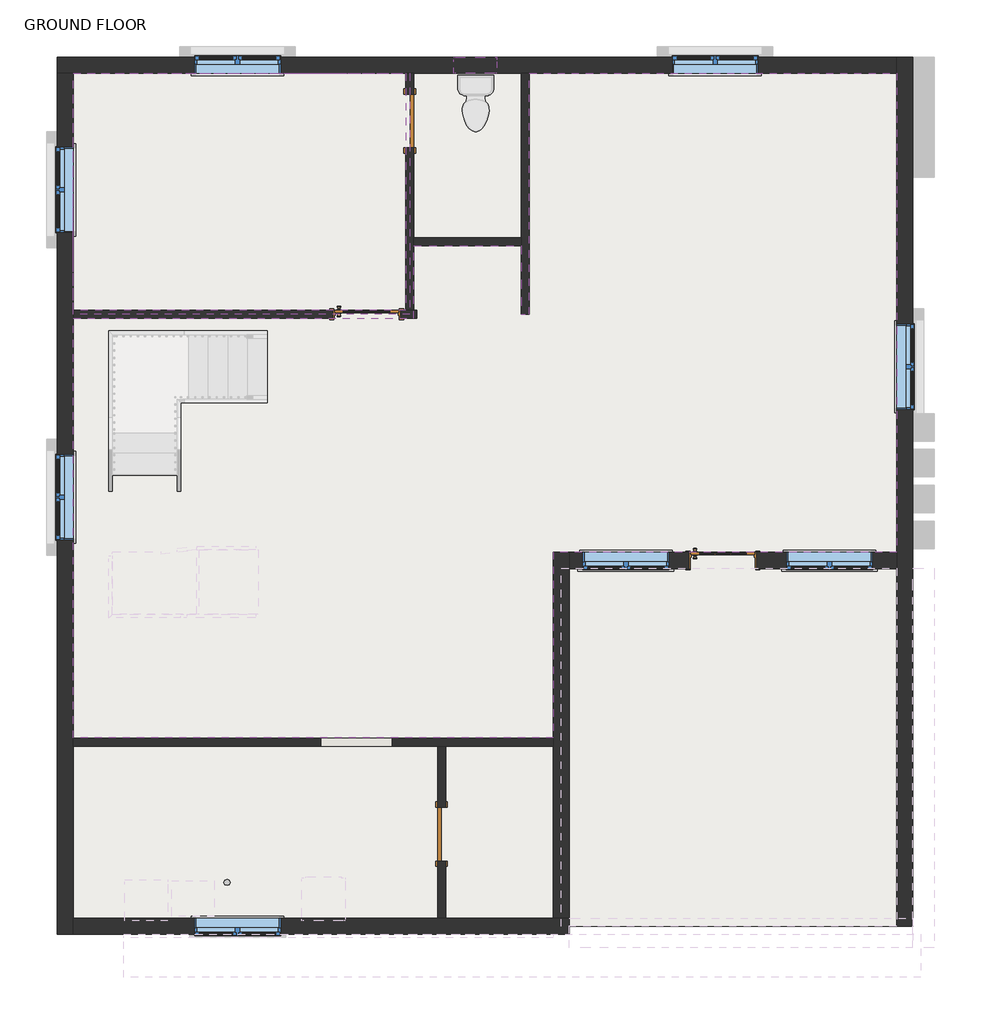
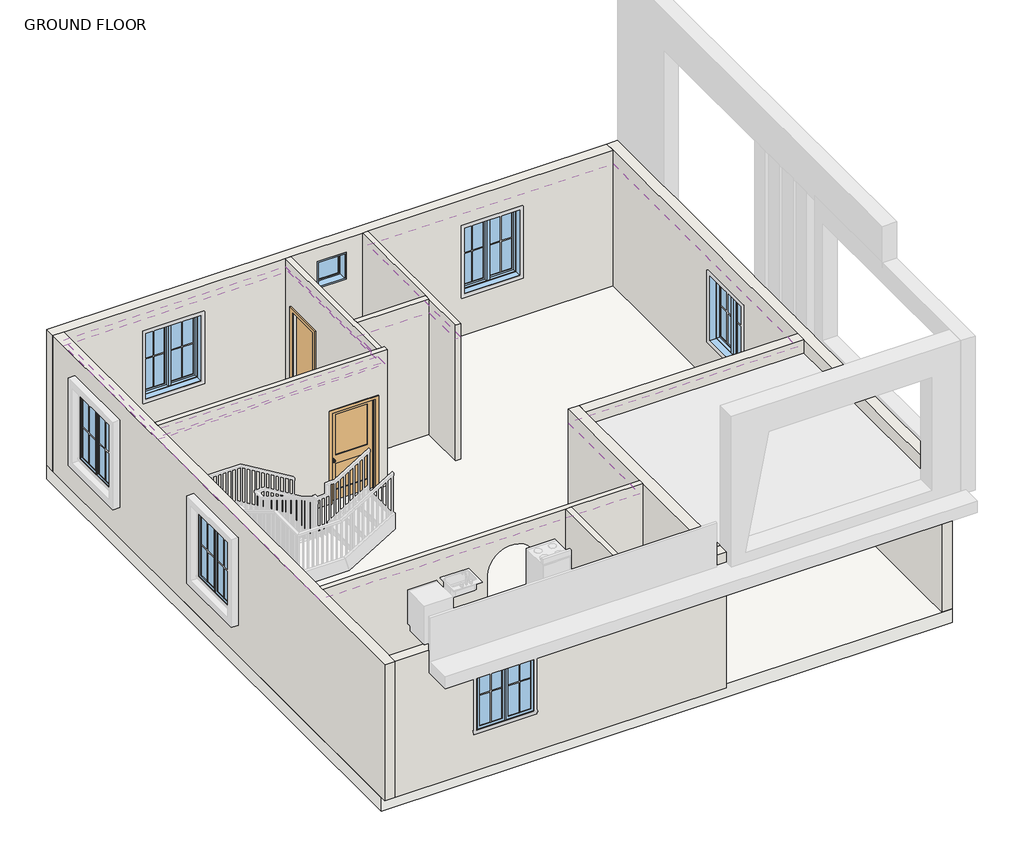
# One storey, part 1 of 4: 12 walls, 9 windows, 4 doors, 3 coverings, 1 slab.
"""IFC4 building model written with IfcOpenShell, lengths in millimetres."""

from ifc_helpers import new_model, si_unit, frame, origin, origin_with_axes, place, context, project, spatial, polyline, circle_curve, outline, extrude, faceted_brep, transform, mapped, element, save
from ifc_brep_helpers import plane_surface, revolved_surface, advanced_brep
from components import door_29124af5, door_c89e1556, door_d8f5dbb5, window_80340324, window_8377141f

model = new_model("IFC4")

# Units and contexts
model_context = context("Model", 3, world=origin())
ifc_project = project(units=[si_unit("LENGTHUNIT", "METRE", prefix="MILLI")], contexts=[model_context])

# Site, building, storey
site = spatial("IfcSite", under=ifc_project)
building = spatial("IfcBuilding", under=site)
storey = spatial("IfcBuildingStorey", under=building, Name="GROUND FLOOR", Elevation=304.8)

# Coverings
placement = place(None, origin())
element("IfcCovering", 1, ObjectType="WHITE CEILING", at=placement, inside=storey, context=model_context, shape_type="SweptSolid", body=[
    extrude(outline(polyline([(-7115.7086008, 4742.0155883), (-7115.7086008, 1389.2155883), (-11821.0586008, 1389.2155883), (-11821.0586008, 4742.0155883), (-7115.7086008, 4742.0155883)])), frame((0.0, 0.0, 3175.0), z_axis=(0.0, 0.0, 1.0), x_axis=(1.0, 0.0, 0.0)), (0.0, 0.0, 1.0), 107.95),
])
element("IfcCovering", 2, ObjectType="WHITE CEILING", at=placement, inside=storey, context=model_context, shape_type="SweptSolid", body=[
    extrude(outline(polyline([(-7058.5586008, 4742.0155883), (-7058.5586008, 1332.0655883), (-11821.0586008, 1332.0655883), (-11821.0586008, 4742.0155883), (-7058.5586008, 4742.0155883)]), holes=[polyline([(-7363.3586008, 4437.2155883), (-11516.2586008, 4437.2155883), (-11516.2586008, 1636.8655883), (-7363.3586008, 1636.8655883), (-7363.3586008, 4437.2155883)])]), frame((0.0, 0.0, 3048.0), z_axis=(0.0, 0.0, 1.0), x_axis=(1.0, 0.0, 0.0)), (0.0, 0.0, 1.0), 107.95),
    extrude(outline(polyline([(-7922.1586008, 3878.4155883), (-7922.1586008, 2195.6655883), (-10957.4586008, 2195.6655883), (-10957.4586008, 3878.4155883), (-7922.1586008, 3878.4155883)]), holes=[polyline([(-7972.9586008, 3827.6155883), (-10906.6586008, 3827.6155883), (-10906.6586008, 2246.4655883), (-7972.9586008, 2246.4655883), (-7972.9586008, 3827.6155883)])]), frame((0.0, 0.0, 3048.0), z_axis=(0.0, 0.0, 1.0), x_axis=(1.0, 0.0, 0.0)), (0.0, 0.0, 1.0), 107.95),
    extrude(outline(polyline([(-8023.7586008, 3776.8155883), (-8023.7586008, 2297.2655883), (-10855.8586008, 2297.2655883), (-10855.8586008, 3776.8155883), (-8023.7586008, 3776.8155883)]), holes=[polyline([(-8074.5586008, 3726.0155883), (-10805.0586008, 3726.0155883), (-10805.0586008, 2348.0655883), (-8074.5586008, 2348.0655883), (-8074.5586008, 3726.0155883)])]), frame((0.0, 0.0, 3048.0), z_axis=(0.0, 0.0, 1.0), x_axis=(1.0, 0.0, 0.0)), (0.0, 0.0, 1.0), 107.95),
    extrude(outline(polyline([(-8125.3586008, 3675.2155883), (-8125.3586008, 2398.8655883), (-10754.2586008, 2398.8655883), (-10754.2586008, 3675.2155883), (-8125.3586008, 3675.2155883)]), holes=[polyline([(-8176.1586008, 3624.4155883), (-10703.4586008, 3624.4155883), (-10703.4586008, 2449.6655883), (-8176.1586008, 2449.6655883), (-8176.1586008, 3624.4155883)])]), frame((0.0, 0.0, 3048.0), z_axis=(0.0, 0.0, 1.0), x_axis=(1.0, 0.0, 0.0)), (0.0, 0.0, 1.0), 107.95),
    extrude(outline(polyline([(-8226.9586008, 3573.6155883), (-8226.9586008, 2500.4655883), (-10652.6586008, 2500.4655883), (-10652.6586008, 3573.6155883), (-8226.9586008, 3573.6155883)]), holes=[polyline([(-8277.7586008, 3522.8155883), (-10601.8586008, 3522.8155883), (-10601.8586008, 2551.2655883), (-8277.7586008, 2551.2655883), (-8277.7586008, 3522.8155883)])]), frame((0.0, 0.0, 3048.0), z_axis=(0.0, 0.0, 1.0), x_axis=(1.0, 0.0, 0.0)), (0.0, 0.0, 1.0), 107.95),
    extrude(outline(polyline([(-8421.7314219, 3141.5453687), (-8421.7314219, 3039.9453687), (-10326.7314219, 3039.9453687), (-10326.7314219, 3141.5453687), (-8421.7314219, 3141.5453687)])), frame((0.0, 0.0, 3048.0), z_axis=(0.0, 0.0, 1.0), x_axis=(1.0, 0.0, 0.0)), (0.0, 0.0, 1.0), 107.95),
    extrude(outline(polyline([(-8421.7314219, 3427.2953687), (-8421.7314219, 3325.6953687), (-10326.7314219, 3325.6953687), (-10326.7314219, 3427.2953687), (-8421.7314219, 3427.2953687)])), frame((0.0, 0.0, 3048.0), z_axis=(0.0, 0.0, 1.0), x_axis=(1.0, 0.0, 0.0)), (0.0, 0.0, 1.0), 107.95),
    extrude(outline(polyline([(-8421.7314219, 2798.6453687), (-8421.7314219, 2697.0453687), (-10326.7314219, 2697.0453687), (-10326.7314219, 2798.6453687), (-8421.7314219, 2798.6453687)])), frame((0.0, 0.0, 3048.0), z_axis=(0.0, 0.0, 1.0), x_axis=(1.0, 0.0, 0.0)), (0.0, 0.0, 1.0), 107.95),
])
element("IfcCovering", 3, ObjectType="WHITE CEILING", at=placement, inside=storey, context=model_context, shape_type="SweptSolid", body=[
    extrude(outline(polyline([(-5363.1086008, 1332.0655883), (-5363.1086008, 4742.0155883), (-162.4586008, 4742.0155883), (-162.4586008, -2039.7844117), (-5026.5586008, -2039.7844117), (-5026.5586008, -4668.6844117), (-11821.0586008, -4668.6844117), (-11821.0586008, 1274.9155883), (-7001.4086008, 1274.9155883), (-7001.4086008, 2303.6155883), (-5477.4086008, 2303.6155883), (-5477.4086008, 1332.0655883), (-5363.1086008, 1332.0655883)]), holes=[polyline([(-9204.4022729, -2001.6844117), (-9236.1522729, -2001.6844117), (-9236.1522729, -1950.8844117), (-10074.3522729, -1950.8844117), (-10302.9522729, -1976.3421011), (-10302.9522729, -132.1404207), (-10302.9522729, 79.9115003), (-9079.7156858, 79.9115003), (-9079.7156858, 130.7115003), (-9079.7156858, 181.5115003), (-9079.7156858, 1045.1115003), (-9079.7156858, 1095.9115003), (-11318.9522729, 1095.9115003), (-11318.9522729, -2966.8844117), (-10213.4567611, -2966.8844117), (-9236.1522729, -2966.8844117), (-9236.1522729, -2916.0844117), (-9204.4022729, -2916.0844117), (-9204.4022729, -2001.6844117)])]), frame((0.0, 0.0, 3048.0), z_axis=(0.0, 0.0, 1.0), x_axis=(1.0, 0.0, 0.0)), (0.0, 0.0, 1.0), 107.95),
])

# Doors
door_shape = door_29124af5(model_context)
element("IfcDoor", 4, ObjectType="Door-Interior-Single-2_Panel-Wood : 36\" x 80\"", at=placement, inside=storey, context=model_context, shape_type="MappedRepresentation", body=[
    mapped(door_shape, transform((-7668.1586008, 1335.2405883, 304.8), x_axis=(1.0, 0.0, 0.0), y_axis=(0.0, 1.0, 0.0), z_axis=(0.0, 0.0, 1.0))),
])
door_2_shape = door_c89e1556(model_context)
element("IfcDoor", 5, ObjectType="Door-Interior-Single-Full Glass-Wood : 36\" x 84\"", at=placement, inside=storey, context=model_context, shape_type="MappedRepresentation", body=[
    mapped(door_2_shape, transform((-2626.2586008, -2150.9094117, 304.8), x_axis=(1.0, 0.0, 0.0), y_axis=(0.0, 1.0, 0.0), z_axis=(0.0, 0.0, 1.0))),
])
door_3_shape = door_d8f5dbb5(model_context)
element("IfcDoor", 6, ObjectType="Single-Flush : 30\" x 80\"", at=placement, inside=storey, context=model_context, shape_type="MappedRepresentation", body=[
    mapped(door_3_shape, transform((-7058.5586008, 4068.9155883, 304.8), x_axis=(0.0, -1.0, 0.0), y_axis=(1.0, 0.0, 0.0), z_axis=(0.0, 0.0, 1.0))),
])
element("IfcDoor", 7, ObjectType="Single-Flush : 30\" x 80\"", at=placement, inside=storey, context=model_context, shape_type="MappedRepresentation", body=[
    mapped(door_3_shape, transform((-6607.7086008, -6030.7594117, 304.8), x_axis=(0.0, 1.0, 0.0), y_axis=(-1.0, 0.0, 0.0), z_axis=(0.0, 0.0, 1.0))),
])

# Slab
element("IfcSlab", 8, ObjectType="MARBLE FLOORING 1'", at=placement, inside=storey, context=model_context, shape_type="SweptSolid", body=[
    extrude(outline(polyline([(66.1413992, 4970.6155883), (66.1413992, -7335.6844117), (-12049.6586008, -7335.6844117), (-12049.6586008, 4970.6155883), (66.1413992, 4970.6155883)])), origin_with_axes(), (0.0, 0.0, 1.0), 304.8),
])

# Walls
element("IfcWall", 9, at=placement, inside=storey, context=model_context, shape_type="Brep", body=[
    faceted_brep([(-7115.7086008, 3687.9155883, 2336.8), (-7115.7086008, 3687.9155883, 304.8), (-7115.7086008, 1389.2155883, 304.8), (-7115.7086008, 1389.2155883, 3352.8), (-7115.7086008, 4742.0155883, 3352.8), (-7115.7086008, 4742.0155883, 304.8), (-7115.7086008, 4449.9155883, 304.8), (-7115.7086008, 4449.9155883, 2336.8), (-7001.4086008, 1389.2155883, 304.8), (-7001.4086008, 2303.6155883, 304.8), (-7001.4086008, 2417.9155883, 304.8), (-7001.4086008, 3687.9155883, 304.8), (-7001.4086008, 3687.9155883, 2336.8), (-7001.4086008, 4449.9155883, 2336.8), (-7001.4086008, 4449.9155883, 304.8), (-7001.4086008, 4742.0155883, 304.8), (-7001.4086008, 4742.0155883, 3352.8), (-7001.4086008, 2417.9155883, 3352.8), (-7001.4086008, 2303.6155883, 3352.8), (-7001.4086008, 1389.2155883, 3352.8)], [[[0, 1, 2, 3, 4, 5, 6, 7]], [[8, 9, 10, 11, 12, 13, 14, 15, 16, 17, 18, 19]], [[6, 5, 15, 14]], [[2, 1, 11, 10, 9, 8]], [[4, 3, 19, 18, 17, 16]], [[5, 4, 16, 15]], [[3, 2, 8, 19]], [[12, 11, 1, 0]], [[13, 12, 0, 7]], [[14, 13, 7, 6]]]),
])
element("IfcWall", 10, at=placement, inside=storey, context=model_context, shape_type="Brep", body=[
    faceted_brep([(-5477.4086008, 4742.0155883, 304.8), (-5477.4086008, 2417.9155883, 304.8), (-5477.4086008, 2303.6155883, 304.8), (-5477.4086008, 1332.0655883, 304.8), (-5477.4086008, 1332.0655883, 3352.8), (-5477.4086008, 2303.6155883, 3352.8), (-5477.4086008, 2417.9155883, 3352.8), (-5477.4086008, 4742.0155883, 3352.8), (-5363.1086008, 4742.0155883, 304.8), (-5363.1086008, 4742.0155883, 3352.8), (-5363.1086008, 1332.0655883, 3352.8), (-5363.1086008, 1332.0655883, 304.8)], [[[0, 1, 2, 3, 4, 5, 6, 7]], [[8, 9, 10, 11]], [[3, 2, 1, 0, 8, 11]], [[4, 3, 11, 10]], [[7, 6, 5, 4, 10, 9]], [[0, 7, 9, 8]]]),
])
element("IfcWall", 11, at=placement, inside=storey, context=model_context, shape_type="Brep", body=[
    faceted_brep([(-6956.9586008, 1274.9155883, 304.8), (-6956.9586008, 1274.9155883, 3352.8), (-11821.0586008, 1274.9155883, 3352.8), (-11821.0586008, 1274.9155883, 304.8), (-8150.7586008, 1274.9155883, 304.8), (-8150.7586008, 1274.9155883, 2362.2), (-7185.5586008, 1274.9155883, 2362.2), (-7185.5586008, 1274.9155883, 304.8), (-6956.9586008, 1389.2155883, 3352.8), (-6956.9586008, 1389.2155883, 304.8), (-7001.4086008, 1389.2155883, 304.8), (-7115.7086008, 1389.2155883, 304.8), (-7185.5586008, 1389.2155883, 304.8), (-7185.5586008, 1389.2155883, 2362.2), (-8150.7586008, 1389.2155883, 2362.2), (-8150.7586008, 1389.2155883, 304.8), (-11821.0586008, 1389.2155883, 304.8), (-11821.0586008, 1389.2155883, 3352.8), (-7115.7086008, 1389.2155883, 3352.8), (-7001.4086008, 1389.2155883, 3352.8)], [[[0, 1, 2, 3, 4, 5, 6, 7]], [[8, 9, 10, 11, 12, 13, 14, 15, 16, 17, 18, 19]], [[9, 0, 7, 12, 11, 10]], [[3, 16, 15, 4]], [[1, 0, 9, 8]], [[2, 1, 8, 19, 18, 17]], [[3, 2, 17, 16]], [[6, 13, 12, 7]], [[13, 6, 5, 14]], [[14, 5, 4, 15]]]),
])
element("IfcWall", 12, at=placement, inside=storey, context=model_context, shape_type="AdvancedBrep", body=[
    advanced_brep(
    [(-11821.0586008, -4782.9844117, 304.8), (-6664.8586008, -4782.9844117, 304.8), (-6550.5586008, -4782.9844117, 304.8), (-5026.5586008, -4782.9844117, 304.8), (-5026.5586008, -4782.9844117, 3352.8), (-6550.5586008, -4782.9844117, 3352.8), (-6664.8586008, -4782.9844117, 3352.8), (-11821.0586008, -4782.9844117, 3352.8), (-7306.1699369, -4782.9844117, 352.7143117), (-8322.1699369, -4782.9844117, 352.7143117), (-8322.1699369, -4782.9844117, 2435.5143117), (-7306.1699369, -4782.9844117, 2435.5143117), (-11821.0586008, -4668.6844117, 304.8), (-11821.0586008, -4668.6844117, 3352.8), (-5026.5586008, -4668.6844117, 3352.8), (-5026.5586008, -4668.6844117, 304.8), (-7306.1699369, -4668.6844117, 352.7143117), (-7306.1699369, -4668.6844117, 2435.5143117), (-8322.1699369, -4668.6844117, 2435.5143117), (-8322.1699369, -4668.6844117, 352.7143117)],
    [
        (0, 1),
        (1, 2),
        (2, 3),
        (3, 4),
        (4, 5),
        (5, 6),
        (6, 7),
        (7, 0),
        (8, 9),
        (9, 10),
        (10, 11, circle_curve(frame((-7814.1699369, -4782.9844117, 2435.5143117), z_axis=(0.0, 1.0, 0.0), x_axis=(-1.0, 0.0, 0.0)), 508.0)),
        (11, 8),
        (12, 13),
        (13, 14),
        (14, 15),
        (15, 12),
        (16, 17),
        (17, 18, circle_curve(frame((-7814.1699369, -4668.6844117, 2435.5143117), z_axis=(0.0, -1.0, 0.0), x_axis=(-1.0, 0.0, 0.0)), 508.0)),
        (18, 19),
        (19, 16),
        (7, 13),
        (12, 0),
        (3, 15),
        (14, 4),
        (8, 16),
        (19, 9),
        (18, 10),
        (17, 11),
    ],
    [
        plane_surface(frame((-11821.0586008, -4782.9844117, 304.8), z_axis=(0.0, -1.0, 0.0), x_axis=(1.0, 0.0, 0.0))),
        plane_surface(frame((-11821.0586008, -4668.6844117, 304.8), z_axis=(0.0, 1.0, 0.0), x_axis=(-1.0, 0.0, 0.0))),
        plane_surface(frame((-11821.0586008, 2722.7155883, 304.8), z_axis=(-1.0, 0.0, 0.0), x_axis=(0.0, 1.0, 0.0))),
        plane_surface(frame((-5026.5586008, -7221.3844117, 304.8), z_axis=(1.0, 0.0, 0.0), x_axis=(0.0, -1.0, 0.0))),
        plane_surface(frame((-11935.3586008, -4782.9844117, 304.8), z_axis=(0.0, 0.0, -1.0), x_axis=(0.0, 1.0, 0.0))),
        plane_surface(frame((-4912.2586008, -4782.9844117, 3352.8), z_axis=(0.0, 0.0, 1.0), x_axis=(0.0, 1.0, 0.0))),
        plane_surface(frame((-7306.1699369, -4782.9844117, 352.7143117), z_axis=(0.0, 0.0, 1.0), x_axis=(0.0, 1.0, 0.0))),
        plane_surface(frame((-8322.1699369, -4782.9844117, 352.7143117), z_axis=(1.0, 0.0, 0.0), x_axis=(0.0, 1.0, 0.0))),
        revolved_surface(polyline([(-8322.1699369, -4668.6844117, 2435.5143117), (-8322.1699369, -4782.9844117, 2435.5143117)]), (-7814.1699369, -4725.8344117, 2435.5143117), (0.0, 1.0, 0.0)),
        plane_surface(frame((-7306.1699369, -4782.9844117, 2435.5143117), z_axis=(-1.0, 0.0, 0.0), x_axis=(0.0, 1.0, 0.0))),
    ],
    [
        (0, [[1, 2, 3, 4, 5, 6, 7, 8], [9, 10, 11, 12]]),
        (1, [[13, 14, 15, 16], [17, 18, 19, 20]]),
        (2, [[-8, 21, -13, 22]]),
        (3, [[-4, 23, -15, 24]]),
        (4, [[-3, -2, -1, -22, -16, -23]]),
        (5, [[-7, -6, -5, -24, -14, -21]]),
        (6, [[-9, 25, -20, 26]]),
        (7, [[-10, -26, -19, 27]]),
        (8, [[-11, -27, -18, 28]]),
        (9, [[-12, -28, -17, -25]]),
    ],
),
])
element("IfcWall", 13, at=placement, inside=storey, context=model_context, shape_type="SweptSolid", body=[
    extrude(outline(polyline([(-4782.9844117, 304.8), (-5649.7594117, 304.8), (-5649.7594117, 2336.8), (-6411.7594117, 2336.8), (-6411.7594117, 304.8), (-7221.3844117, 304.8), (-7221.3844117, 3352.8), (-4782.9844117, 3352.8), (-4782.9844117, 304.8)])), frame((-6664.8586008, 0.0, 0.0), z_axis=(1.0, 0.0, 0.0), x_axis=(0.0, 1.0, 0.0)), (0.0, 0.0, 1.0), 114.3),
])
element("IfcWall", 14, at=placement, inside=storey, context=model_context, shape_type="SweptSolid", body=[
    extrude(outline(polyline([(-7001.4086008, 2417.9155883), (-5477.4086008, 2417.9155883), (-5477.4086008, 2303.6155883), (-7001.4086008, 2303.6155883), (-7001.4086008, 2417.9155883)])), frame((0.0, 0.0, 304.8), z_axis=(0.0, 0.0, 1.0), x_axis=(1.0, 0.0, 0.0)), (0.0, 0.0, 1.0), 3048.0),
])
element("IfcWall", 15, ObjectType="OUTER WALL CREAM WHITE 9\"", at=placement, inside=storey, context=model_context, shape_type="Brep", body=[
    faceted_brep([(-12049.6586008, 4742.0155883, 304.8), (-11821.0586008, 4742.0155883, 304.8), (-7115.7086008, 4742.0155883, 304.8), (-7001.4086008, 4742.0155883, 304.8), (-5477.4086008, 4742.0155883, 304.8), (-5363.1086008, 4742.0155883, 304.8), (-162.4586008, 4742.0155883, 304.8), (-162.4586008, 4742.0155883, 3352.8), (-5363.1086008, 4742.0155883, 3352.8), (-5477.4086008, 4742.0155883, 3352.8), (-7001.4086008, 4742.0155883, 3352.8), (-7115.7086008, 4742.0155883, 3352.8), (-11821.0586008, 4742.0155883, 3352.8), (-12049.6586008, 4742.0155883, 3352.8), (-8887.3586008, 4742.0155883, 2743.2), (-8887.3586008, 4742.0155883, 1219.2), (-10106.5586008, 4742.0155883, 1219.2), (-10106.5586008, 4742.0155883, 2743.2), (-2124.6086008, 4742.0155883, 2743.2), (-2124.6086008, 4742.0155883, 1219.2), (-3343.8086008, 4742.0155883, 1219.2), (-3343.8086008, 4742.0155883, 2743.2), (-5826.6586008, 4742.0155883, 3048.0), (-5826.6586008, 4742.0155883, 2438.4), (-6436.2586008, 4742.0155883, 2438.4), (-6436.2586008, 4742.0155883, 3048.0), (-12049.6586008, 4970.6155883, 304.8), (-12049.6586008, 4970.6155883, 3352.8), (-162.4586008, 4970.6155883, 3352.8), (-162.4586008, 4970.6155883, 304.8), (-8887.3586008, 4970.6155883, 2743.2), (-10106.5586008, 4970.6155883, 2743.2), (-10106.5586008, 4970.6155883, 1219.2), (-8887.3586008, 4970.6155883, 1219.2), (-2124.6086008, 4970.6155883, 2743.2), (-3343.8086008, 4970.6155883, 2743.2), (-3343.8086008, 4970.6155883, 1219.2), (-2124.6086008, 4970.6155883, 1219.2), (-5826.6586008, 4970.6155883, 3048.0), (-6436.2586008, 4970.6155883, 3048.0), (-6436.2586008, 4970.6155883, 2438.4), (-5826.6586008, 4970.6155883, 2438.4)], [[[0, 1, 2, 3, 4, 5, 6, 7, 8, 9, 10, 11, 12, 13], [14, 15, 16, 17], [18, 19, 20, 21], [22, 23, 24, 25]], [[26, 27, 28, 29], [30, 31, 32, 33], [34, 35, 36, 37], [38, 39, 40, 41]], [[6, 5, 4, 3, 2, 1, 0, 26, 29]], [[13, 12, 11, 10, 9, 8, 7, 28, 27]], [[0, 13, 27, 26]], [[7, 6, 29, 28]], [[15, 14, 30, 33]], [[16, 15, 33, 32]], [[17, 16, 32, 31]], [[14, 17, 31, 30]], [[19, 18, 34, 37]], [[20, 19, 37, 36]], [[21, 20, 36, 35]], [[18, 21, 35, 34]], [[23, 22, 38, 41]], [[24, 23, 41, 40]], [[25, 24, 40, 39]], [[22, 25, 39, 38]]]),
])
element("IfcWall", 16, ObjectType="OUTER WALL CREAM WHITE 9\"", at=placement, inside=storey, context=model_context, shape_type="Brep", body=[
    faceted_brep([(-11821.0586008, -7449.9844117, 304.8), (-11821.0586008, -7221.3844117, 304.8), (-11821.0586008, -4782.9844117, 304.8), (-11821.0586008, -4668.6844117, 304.8), (-11821.0586008, 1274.9155883, 304.8), (-11821.0586008, 1389.2155883, 304.8), (-11821.0586008, 4742.0155883, 304.8), (-11821.0586008, 4742.0155883, 3352.8), (-11821.0586008, 1389.2155883, 3352.8), (-11821.0586008, 1274.9155883, 3352.8), (-11821.0586008, -4668.6844117, 3352.8), (-11821.0586008, -4782.9844117, 3352.8), (-11821.0586008, -7221.3844117, 3352.8), (-11821.0586008, -7449.9844117, 3352.8), (-11821.0586008, 3703.7905883, 2743.2), (-11821.0586008, 3703.7905883, 1219.2), (-11821.0586008, 2484.5905883, 1219.2), (-11821.0586008, 2484.5905883, 2743.2), (-11821.0586008, -649.1344117, 2743.2), (-11821.0586008, -649.1344117, 1219.2), (-11821.0586008, -1868.3344117, 1219.2), (-11821.0586008, -1868.3344117, 2743.2), (-12049.6586008, -7449.9844117, 304.8), (-12049.6586008, -7449.9844117, 3352.8), (-12049.6586008, 4742.0155883, 3352.8), (-12049.6586008, 4742.0155883, 304.8), (-12049.6586008, 3703.7905883, 2743.2), (-12049.6586008, 2484.5905883, 2743.2), (-12049.6586008, 2484.5905883, 1219.2), (-12049.6586008, 3703.7905883, 1219.2), (-12049.6586008, -649.1344117, 2743.2), (-12049.6586008, -1868.3344117, 2743.2), (-12049.6586008, -1868.3344117, 1219.2), (-12049.6586008, -649.1344117, 1219.2)], [[[0, 1, 2, 3, 4, 5, 6, 7, 8, 9, 10, 11, 12, 13], [14, 15, 16, 17], [18, 19, 20, 21]], [[22, 23, 24, 25], [26, 27, 28, 29], [30, 31, 32, 33]], [[6, 5, 4, 3, 2, 1, 0, 22, 25]], [[13, 12, 11, 10, 9, 8, 7, 24, 23]], [[0, 13, 23, 22]], [[7, 6, 25, 24]], [[15, 14, 26, 29]], [[16, 15, 29, 28]], [[17, 16, 28, 27]], [[14, 17, 27, 26]], [[19, 18, 30, 33]], [[20, 19, 33, 32]], [[21, 20, 32, 31]], [[18, 21, 31, 30]]]),
])
element("IfcWall", 17, ObjectType="OUTER WALL CREAM WHITE 9\"", at=placement, inside=storey, context=model_context, shape_type="Brep", body=[
    faceted_brep([(-4797.9586008, -7221.3844117, 304.8), (-5026.5586008, -7221.3844117, 304.8), (-6550.5586008, -7221.3844117, 304.8), (-6664.8586008, -7221.3844117, 304.8), (-11821.0586008, -7221.3844117, 304.8), (-11821.0586008, -7221.3844117, 3352.8), (-6664.8586008, -7221.3844117, 3352.8), (-6550.5586008, -7221.3844117, 3352.8), (-5026.5586008, -7221.3844117, 3352.8), (-4797.9586008, -7221.3844117, 3352.8), (-10106.5586008, -7221.3844117, 2743.2), (-10106.5586008, -7221.3844117, 1219.2), (-8887.3586008, -7221.3844117, 1219.2), (-8887.3586008, -7221.3844117, 2743.2), (-4797.9586008, -7449.9844117, 304.8), (-4797.9586008, -7449.9844117, 3352.8), (-11821.0586008, -7449.9844117, 3352.8), (-11821.0586008, -7449.9844117, 304.8), (-10106.5586008, -7449.9844117, 2743.2), (-8887.3586008, -7449.9844117, 2743.2), (-8887.3586008, -7449.9844117, 1219.2), (-10106.5586008, -7449.9844117, 1219.2)], [[[0, 1, 2, 3, 4, 5, 6, 7, 8, 9], [10, 11, 12, 13]], [[14, 15, 16, 17], [18, 19, 20, 21]], [[4, 3, 2, 1, 0, 14, 17]], [[9, 8, 7, 6, 5, 16, 15]], [[5, 4, 17, 16]], [[0, 9, 15, 14]], [[11, 10, 18, 21]], [[12, 11, 21, 20]], [[13, 12, 20, 19]], [[10, 13, 19, 18]]]),
])
element("IfcWall", 18, ObjectType="OUTER WALL CREAM WHITE 9\"", at=placement, inside=storey, context=model_context, shape_type="Brep", body=[
    faceted_brep([(-162.4586008, 4970.6155883, 304.8), (-162.4586008, 4742.0155883, 304.8), (-162.4586008, -2039.7844117, 304.8), (-162.4586008, -2268.3844117, 304.8), (-162.4586008, -7335.6844117, 304.8), (-162.4586008, -7335.6844117, 3352.8), (-162.4586008, -2268.3844117, 3352.8), (-162.4586008, -2039.7844117, 3352.8), (-162.4586008, 4742.0155883, 3352.8), (-162.4586008, 4970.6155883, 3352.8), (-162.4586008, -20.4844117, 2743.2), (-162.4586008, -20.4844117, 1219.2), (-162.4586008, 1198.7155883, 1219.2), (-162.4586008, 1198.7155883, 2743.2), (66.1413992, 4970.6155883, 304.8), (66.1413992, 4970.6155883, 3352.8), (66.1413992, -7335.6844117, 3352.8), (66.1413992, -7335.6844117, 304.8), (66.1413992, -20.4844117, 2743.2), (66.1413992, 1198.7155883, 2743.2), (66.1413992, 1198.7155883, 1219.2), (66.1413992, -20.4844117, 1219.2)], [[[0, 1, 2, 3, 4, 5, 6, 7, 8, 9], [10, 11, 12, 13]], [[14, 15, 16, 17], [18, 19, 20, 21]], [[4, 3, 2, 1, 0, 14, 17]], [[5, 4, 17, 16]], [[9, 8, 7, 6, 5, 16, 15]], [[0, 9, 15, 14]], [[11, 10, 18, 21]], [[12, 11, 21, 20]], [[13, 12, 20, 19]], [[10, 13, 19, 18]]]),
])
element("IfcWall", 19, ObjectType="OUTER WALL CREAM WHITE 9\"", at=placement, inside=storey, context=model_context, shape_type="Brep", body=[
    faceted_brep([(-4797.9586008, -7221.3844117, 304.8), (-4797.9586008, -2268.3844117, 304.8), (-4797.9586008, -2039.7844117, 304.8), (-4797.9586008, -2039.7844117, 3352.8), (-4797.9586008, -2268.3844117, 3352.8), (-4797.9586008, -7221.3844117, 3352.8), (-5026.5586008, -7221.3844117, 304.8), (-5026.5586008, -7221.3844117, 3352.8), (-5026.5586008, -4782.9844117, 3352.8), (-5026.5586008, -4668.6844117, 3352.8), (-5026.5586008, -2039.7844117, 3352.8), (-5026.5586008, -2039.7844117, 304.8), (-5026.5586008, -4668.6844117, 304.8), (-5026.5586008, -4782.9844117, 304.8)], [[[0, 1, 2, 3, 4, 5]], [[6, 7, 8, 9, 10, 11, 12, 13]], [[2, 1, 0, 6, 13, 12, 11]], [[5, 4, 3, 10, 9, 8, 7]], [[3, 2, 11, 10]], [[0, 5, 7, 6]]]),
])
element("IfcWall", 20, ObjectType="OUTER WALL CREAM WHITE 9\"", at=placement, inside=storey, context=model_context, shape_type="SweptSolid", body=[
    extrude(outline(polyline([(3352.8, -162.4586008), (3352.8, -4797.9586008), (304.8, -4797.9586008), (304.8, -3108.8586008), (2463.8, -3108.8586008), (2463.8, -2143.6586008), (304.8, -2143.6586008), (304.8, -162.4586008), (3352.8, -162.4586008)]), holes=[polyline([(2743.2, -1724.5586008), (2743.2, -505.3586008), (1219.2, -505.3586008), (1219.2, -1724.5586008), (2743.2, -1724.5586008)]), polyline([(2743.2, -4607.4586008), (2743.2, -3388.2586008), (1219.2, -3388.2586008), (1219.2, -4607.4586008), (2743.2, -4607.4586008)])]), frame((0.0, -2268.3844117, 0.0), z_axis=(0.0, 1.0, 0.0), x_axis=(0.0, 0.0, 1.0)), (0.0, 0.0, 1.0), 228.6),
])

# Windows
window_shape = window_80340324(model_context)
element("IfcWindow", 21, ObjectType="Fixed : 24\" x 24\"", at=placement, inside=storey, context=model_context, shape_type="MappedRepresentation", body=[
    mapped(window_shape, transform((-6093.3586008, 4856.3155883, 1524.0), x_axis=(1.0, 0.0, 0.0), y_axis=(0.0, 1.0, 0.0), z_axis=(0.0, 0.0, 1.0))),
])
window_2_shape = window_8377141f(model_context)
element("IfcWindow", 22, ObjectType="Window-Casement-Double : BLACK MATERIAL 2\"", at=placement, inside=storey, context=model_context, shape_type="MappedRepresentation", body=[
    mapped(window_2_shape, transform((-1114.9586008, -2154.0844117, 304.8), x_axis=(-1.0, 0.0, 0.0), y_axis=(0.0, -1.0, 0.0), z_axis=(0.0, 0.0, 1.0))),
])
element("IfcWindow", 23, ObjectType="Window-Casement-Double : BLACK MATERIAL 2\"", at=placement, inside=storey, context=model_context, shape_type="MappedRepresentation", body=[
    mapped(window_2_shape, transform((-3997.8586008, -2154.0844117, 304.8), x_axis=(-1.0, 0.0, 0.0), y_axis=(0.0, -1.0, 0.0), z_axis=(0.0, 0.0, 1.0))),
])
element("IfcWindow", 24, ObjectType="Window-Casement-Double : BLACK MATERIAL 2\"", at=placement, inside=storey, context=model_context, shape_type="MappedRepresentation", body=[
    mapped(window_2_shape, transform((-9496.9586008, -7335.6844117, 304.8), x_axis=(-1.0, 0.0, 0.0), y_axis=(0.0, -1.0, 0.0), z_axis=(0.0, 0.0, 1.0))),
])
element("IfcWindow", 25, ObjectType="Window-Casement-Double : BLACK MATERIAL 2\"", at=placement, inside=storey, context=model_context, shape_type="MappedRepresentation", body=[
    mapped(window_2_shape, transform((-48.1586008, 589.1155883, 304.8), x_axis=(0.0, -1.0, 0.0), y_axis=(1.0, 0.0, 0.0), z_axis=(0.0, 0.0, 1.0))),
])
element("IfcWindow", 26, ObjectType="Window-Casement-Double : BLACK MATERIAL 2\"", at=placement, inside=storey, context=model_context, shape_type="MappedRepresentation", body=[
    mapped(window_2_shape, transform((-9496.9586008, 4856.3155883, 304.8), x_axis=(1.0, 0.0, 0.0), y_axis=(0.0, 1.0, 0.0), z_axis=(0.0, 0.0, 1.0))),
])
element("IfcWindow", 27, ObjectType="Window-Casement-Double : BLACK MATERIAL 2\"", at=placement, inside=storey, context=model_context, shape_type="MappedRepresentation", body=[
    mapped(window_2_shape, transform((-11935.3586008, 3094.1905883, 304.8), x_axis=(0.0, 1.0, 0.0), y_axis=(-1.0, 0.0, 0.0), z_axis=(0.0, 0.0, 1.0))),
])
element("IfcWindow", 28, ObjectType="Window-Casement-Double : BLACK MATERIAL 2\"", at=placement, inside=storey, context=model_context, shape_type="MappedRepresentation", body=[
    mapped(window_2_shape, transform((-11935.3586008, -1258.7344117, 304.8), x_axis=(0.0, 1.0, 0.0), y_axis=(-1.0, 0.0, 0.0), z_axis=(0.0, 0.0, 1.0))),
])
element("IfcWindow", 29, ObjectType="Window-Casement-Double : BLACK MATERIAL 2\"", at=placement, inside=storey, context=model_context, shape_type="MappedRepresentation", body=[
    mapped(window_2_shape, transform((-2734.2086008, 4856.3155883, 304.8), x_axis=(1.0, 0.0, 0.0), y_axis=(0.0, 1.0, 0.0), z_axis=(0.0, 0.0, 1.0))),
])

save(model, "model.ifc")

# Revit data of these elements
# Type "WHITE CEILING"
#   Assembly Code = "C3030220"
#   built-in parameter 1002203 = 1 (stored number, unit not read)
#   built-in parameter 1002202 = 1 (stored number, unit not read)
#   Layers, outside or top first: 0' - 3 5/8" "WHITE CEILING" (function 1); 0' - 0 5/8" "WHITE CEILING" (function 5)
# Type "Door-Interior-Single-2_Panel-Wood : 36\" x 80\""
#   Type Mark = "9"
#   Assembly Code = "C1020300"
#   Analytic Construction = "Wooden"
#   Top Rail = 0' - 4 11/16"
#   Thickness = 0' - 1 3/8"
#   Thermal Resistance (R) = 2.5876 (h·ft²·°F)/BTU
#   Swing Angle [instance default] = 90.00°
#   Stiles = 0' - 4 3/4"
#   Rough Width = 3' - 2"
#   Rough Height = 6' - 9"
#   Lock Rail = 0' - 7 1/2"
#   Height = 6' - 8"
#   Width = 3' - 0"
#   Heat Transfer Coefficient (U) = 0.3865 BTU/(h·ft²·°F)
#   Bottom Rail = 0' - 9 1/8"
#   Trim Material = Cherry
#   Panel Material = Cherry
#   Frame Material = Cherry
#   Door Handle Material = Aluminum
#   Visual Light Transmittance = 0
#   Solar Heat Gain Coefficient = 0
#   Wall Closure = (empty or 0)
#   Function = (empty or 0)
# Type "Door-Interior-Single-Full Glass-Wood : 36\" x 84\""
#   Type Mark = "8"
#   Assembly Code = "C1020300"
#   Analytic Construction = "Wood frame with single clear glass"
#   Top Rail = 0' - 4 11/16"
#   Thickness = 0' - 1 3/8"
#   Thermal Resistance (R) = 1.0102 (h·ft²·°F)/BTU
#   Swing Angle [instance default] = 90.00°
#   Stiles = 0' - 4 3/4"
#   Rough Width = 3' - 2"
#   Rough Height = 7' - 1"
#   Height = 7' - 0"
#   Width = 3' - 0"
#   Heat Transfer Coefficient (U) = 0.9900 BTU/(h·ft²·°F)
#   Bottom Rail = 0' - 9 1/8"
#   Show Grill [instance default] = yes
#   Trim Material = Cherry
#   Panel Material = Cherry
#   Frame Material = Cherry
#   Door Handle Material = Aluminum
#   Visual Light Transmittance = 0
#   Solar Heat Gain Coefficient = 0
#   Wall Closure = (empty or 0)
#   Function = (empty or 0)
# Type "Single-Flush : 30\" x 80\""
#   Type Mark = "5"
#   Construction Type Id = "MDOOR"
#   Assembly Code = "C1020"
#   Analytic Construction = "Metal"
#   Thickness = 0' - 2"
#   Heat Transfer Coefficient (U) = 0.651978 BTU/(h·ft²·°F)
#   Height = 6' - 8"
#   Trim Projection Ext = 0' - 1"
#   Trim Projection Int = 0' - 1"
#   Trim Width = 0' - 3"
#   Width = 2' - 6"
#   Define Thermal Properties by = 1
#   Define Thermal Properties by = 1
#   Door Material = Door - Panel
#   Frame Material = Door - Frame
#   Visual Light Transmittance = 0
#   Solar Heat Gain Coefficient = 0
#   Function = (empty or 0)
#   Wall Closure = (empty or 0)
# Type "MARBLE FLOORING 1'"
#   Assembly Code = "B1010"
#   Function = 0
#   Layers, outside or top first: 1' - 0" "MARBLE MATERIAL" (function 1)
# Type
#   Assembly Code = "B2010"
#   Layers, outside or top first: 0' - 4 1/2" "OFF WHITE COLOUR" (function 1)
# Type "OUTER WALL CREAM WHITE 9\""
#   Assembly Code = "B2010"
#   Layers, outside or top first: 0' - 9" "OFF WHITE COLOUR" (function 1)
# Type "Fixed : 24\" x 24\""
#   Type Mark = "3"
#   Construction Type Id = "GSP4R"
#   Assembly Code = "B2020100"
#   Analytic Construction = "1/8 in Pilkington single glazing"
#   Visual Light Transmittance = 0.9
#   Solar Heat Gain Coefficient = 0.78
#   Heat Transfer Coefficient (U) = 0.6496 BTU/(h·ft²·°F)
#   Height = 2' - 0"
#   Default Sill Height = 3' - 0"
#   Width = 2' - 0"
#   Window Inset = 0' - 0 3/4"
#   Define Thermal Properties by = 1
#   Define Thermal Properties by = 1
#   Glass Pane Material = Glass
#   Sash Material = Sash
#   Wall Closure = (empty or 0)
# Type "Window-Casement-Double : BLACK MATERIAL 2\""
#   Type Mark = "18"
#   Fire Rating = "0.5h"
#   Assembly Code = "B2020100"
#   Analytic Construction = "Double glazing - domestic"
#   Frame Extension [instance default] = 0' - 0 1/4"
#   Window Inset [instance default] = 0' - 0"
#   Wall Thickness [instance default] = 0' - 6"
#   Interior Wall Closure [instance default] = 0' - 2 1/4"
#   Half Width = 2' - 0"
#   Visual Light Transmittance = 0.81
#   Thermal Resistance (R) = 1.8146 (h·ft²·°F)/BTU
#   Solar Heat Gain Coefficient = 0.76
#   Rough Width = 4' - 0 1/2"
#   Rough Height = 5' - 0 1/2"
#   Height = 5' - 0"
#   Heat Transfer Coefficient (U) = 0.5511 BTU/(h·ft²·°F)
#   Exterior Wall Closure [instance default] = 0' - 1 1/4"
#   Extension Jamb [instance default] = 0' - 2 1/4"
#   Default Sill Height = 3' - 0"
#   Width = 4' - 0"
#   Muntin Visibility = yes
#   Interior Trim Visibility [instance default] = yes
#   Exterior Trim Visibility [instance default] = yes
#   Extension Jamb Visibility [instance default] = yes
#   Interior Trim Material = Wood - Stained
#   Muntin Pattern = Muntin Pattern_2x2 : Muntin Pattern_2x2
#   Interior Trim = Trim-Window-Interior-Flat : Picture Frame
#   Interior Frame Material = Wood - Stained
#   Glass Panel Material = Glass
#   Exterior Trim Material = BLACK MATERIAL
#   Exterior Trim = Trim-Window-Exterior-Flat : with Sill
#   Exterior Frame Material = BLACK MATERIAL
#   Wall Closure = (empty or 0)
# Element 1 (IfcCovering, "WHITE CEILING")
#   Height Offset From Level = 9' - 5"
#   Phase Created = New Construction
#   Materials on its faces: "WHITE CEILING"
# Elements 2, 3 (IfcCovering, "WHITE CEILING")
#   Height Offset From Level = 9' - 0"
#   Phase Created = New Construction
#   Materials on its faces: "WHITE CEILING"
# Element 4 (IfcDoor, "Door-Interior-Single-2_Panel-Wood : 36\" x 80\"")
#   Swing Angle = 90.00°
#   Phase Created = New Construction
#   Materials on its faces: "Cherry", "Aluminum"
# Element 5 (IfcDoor, "Door-Interior-Single-Full Glass-Wood : 36\" x 84\"")
#   Swing Angle = 90.00°
#   Show Grill = yes
#   Phase Created = New Construction
#   Materials on its faces: "Cherry", "Aluminum", "Glass"
# Elements 6, 7 (IfcDoor, "Single-Flush : 30\" x 80\"")
#   Phase Created = New Construction
#   Materials on its faces: "Door - Frame", "Door - Panel"
# Element 8 (IfcSlab, "MARBLE FLOORING 1'")
#   Height Offset From Level = 0' - 0"
#   Phase Created = New Construction
#   Materials on its faces: "MARBLE MATERIAL"
# Elements 9, 10, 11, 12, 13, 14 (IfcWall)
#   Top Offset = 0' - 0"
#   Base Offset = 0' - 0"
#   wall height = 10' - 0"
#   Phase Created = New Construction
#   Base Constraint = GROUND FLOOR
#   Top Constraint = FIRST FLOOR
#   Materials on its faces: "OFF WHITE COLOUR"
# Elements 15, 16, 17, 18, 19, 20 (IfcWall, "OUTER WALL CREAM WHITE 9\"")
#   Top Offset = 0' - 0"
#   Base Offset = 0' - 0"
#   wall height = 10' - 0"
#   Phase Created = New Construction
#   Base Constraint = GROUND FLOOR
#   Top Constraint = FIRST FLOOR
#   Materials on its faces: "OFF WHITE COLOUR"
# Element 21 (IfcWindow, "Fixed : 24\" x 24\"")
#   Mark = "9"
#   Phase Created = New Construction
#   Materials on its faces: "Sash", "Glass"
# Element 22 (IfcWindow, "Window-Casement-Double : BLACK MATERIAL 2\"")
#   Mark = "1"
#   Window Inset = 0' - 0"
#   Interior Wall Closure = 0' - 2 1/4"
#   Frame Extension = 0' - 0 1/4"
#   Exterior Wall Closure = 0' - 1 1/4"
#   Interior Trim Visibility = yes
#   Exterior Trim Visibility = yes
#   Phase Created = New Construction
#   Materials on its faces: "Wood - Stained", "Glass", "BLACK MATERIAL"
# Element 23 (IfcWindow, "Window-Casement-Double : BLACK MATERIAL 2\"")
#   Mark = "2"
#   Window Inset = 0' - 0"
#   Interior Wall Closure = 0' - 2 1/4"
#   Frame Extension = 0' - 0 1/4"
#   Exterior Wall Closure = 0' - 1 1/4"
#   Interior Trim Visibility = yes
#   Exterior Trim Visibility = yes
#   Phase Created = New Construction
#   Materials on its faces: "Wood - Stained", "Glass", "BLACK MATERIAL"
# Element 24 (IfcWindow, "Window-Casement-Double : BLACK MATERIAL 2\"")
#   Mark = "3"
#   Window Inset = 0' - 0"
#   Interior Wall Closure = 0' - 2 1/4"
#   Frame Extension = 0' - 0 1/4"
#   Exterior Wall Closure = 0' - 1 1/4"
#   Interior Trim Visibility = yes
#   Exterior Trim Visibility = yes
#   Phase Created = New Construction
#   Materials on its faces: "Wood - Stained", "Glass", "BLACK MATERIAL"
# Element 25 (IfcWindow, "Window-Casement-Double : BLACK MATERIAL 2\"")
#   Mark = "4"
#   Window Inset = 0' - 0"
#   Interior Wall Closure = 0' - 2 1/4"
#   Frame Extension = 0' - 0 1/4"
#   Exterior Wall Closure = 0' - 1 1/4"
#   Interior Trim Visibility = yes
#   Exterior Trim Visibility = yes
#   Phase Created = New Construction
#   Materials on its faces: "Wood - Stained", "Glass", "BLACK MATERIAL"
# Element 26 (IfcWindow, "Window-Casement-Double : BLACK MATERIAL 2\"")
#   Mark = "5"
#   Window Inset = 0' - 0"
#   Interior Wall Closure = 0' - 2 1/4"
#   Frame Extension = 0' - 0 1/4"
#   Exterior Wall Closure = 0' - 1 1/4"
#   Interior Trim Visibility = yes
#   Exterior Trim Visibility = yes
#   Phase Created = New Construction
#   Materials on its faces: "Wood - Stained", "Glass", "BLACK MATERIAL"
# Element 27 (IfcWindow, "Window-Casement-Double : BLACK MATERIAL 2\"")
#   Mark = "6"
#   Window Inset = 0' - 0"
#   Interior Wall Closure = 0' - 2 1/4"
#   Frame Extension = 0' - 0 1/4"
#   Exterior Wall Closure = 0' - 1 1/4"
#   Interior Trim Visibility = yes
#   Exterior Trim Visibility = yes
#   Phase Created = New Construction
#   Materials on its faces: "Wood - Stained", "Glass", "BLACK MATERIAL"
# Element 28 (IfcWindow, "Window-Casement-Double : BLACK MATERIAL 2\"")
#   Mark = "7"
#   Window Inset = 0' - 0"
#   Interior Wall Closure = 0' - 2 1/4"
#   Frame Extension = 0' - 0 1/4"
#   Exterior Wall Closure = 0' - 1 1/4"
#   Interior Trim Visibility = yes
#   Exterior Trim Visibility = yes
#   Phase Created = New Construction
#   Materials on its faces: "Wood - Stained", "Glass", "BLACK MATERIAL"
# Element 29 (IfcWindow, "Window-Casement-Double : BLACK MATERIAL 2\"")
#   Mark = "8"
#   Window Inset = 0' - 0"
#   Interior Wall Closure = 0' - 2 1/4"
#   Frame Extension = 0' - 0 1/4"
#   Exterior Wall Closure = 0' - 1 1/4"
#   Interior Trim Visibility = yes
#   Exterior Trim Visibility = yes
#   Phase Created = New Construction
#   Materials on its faces: "Wood - Stained", "Glass", "BLACK MATERIAL"
# Materials
#   "WHITE CEILING": class "Generic", colour RGB 120 120 120, transparency 0, Cost = 0
#   "Cherry": class "Wood", colour RGB 226 177 128, transparency 0, Description = "Prunus Serotina", Cost = 0
#   "Aluminum": class "Metal", colour RGB 247 247 247, transparency 0, Description = "Aluminum 6061", Cost = 0
#   "Door - Panel": class "Wood", colour RGB 210 159 95, transparency 0, Cost = 0
#   "Door - Frame": colour RGB 118 70 51, transparency 0, Cost = 0
#   "MARBLE MATERIAL": class "Generic", colour RGB 120 120 120, transparency 0, Cost = 0
#   "OFF WHITE COLOUR": class "Generic", colour RGB 120 120 120, transparency 0, Cost = 0
#   "Glass": class "Glass", colour RGB 0 128 192, transparency 0.75, Description = "Soda Lime Glass", Cost = 0
#   "Sash": class "Wood", colour RGB 224 178 126, transparency 0, Cost = 0
#   "Wood - Stained": class "Wood", colour RGB 224 178 126, transparency 0, Cost = 0
#   "BLACK MATERIAL": class "Generic", colour RGB 120 120 120, transparency 0, Cost = 0
# Room at (-9496.959, 3094.191) mm, phase "New Construction", upper level "GROUND FLOOR", upper offset 10' - 0", lower offset 0' - 0"
#   Number = "1"
#   Name = "BEDROOM"
# Room at (-9271.534, -6030.759) mm, phase "New Construction", upper level "GROUND FLOOR", upper offset 10' - 0", lower offset 0' - 0"
#   Number = "2"
#   Name = "KITCHEN ROOM"
# Room at (-5759.984, -6030.759) mm, phase "New Construction", upper level "GROUND FLOOR", upper offset 10' - 0", lower offset 0' - 0"
#   Number = "3"
#   Name = "STORE"
# Room at (-6239.409, 3608.541) mm, phase "New Construction", upper level "GROUND FLOOR", upper offset 10' - 0", lower offset 0' - 0"
#   Number = "4"
#   Name = "TOILET"
# Room at (-6239.409, 1817.841) mm, phase "New Construction", upper level "GROUND FLOOR", upper offset 10' - 0", lower offset 0' - 0"
#   Number = "5"
# Room at (-8423.809, -1696.884) mm, phase "New Construction", upper level "GROUND FLOOR", upper offset 10' - 0", lower offset 0' - 0"
#   Number = "6"
#   Name = "DINING ROOM"
# Room at (-2762.784, 1351.116) mm, phase "New Construction", upper level "GROUND FLOOR", upper offset 10' - 0", lower offset 0' - 0"
#   Number = "7"
#   Name = "LIVING ROOM"
# Room at (-2480.209, -4744.884) mm, phase "New Construction", upper level "GROUND FLOOR", upper offset 10' - 0", lower offset 0' - 0"
#   Number = "8"
#   Name = "PARKING AREA"
